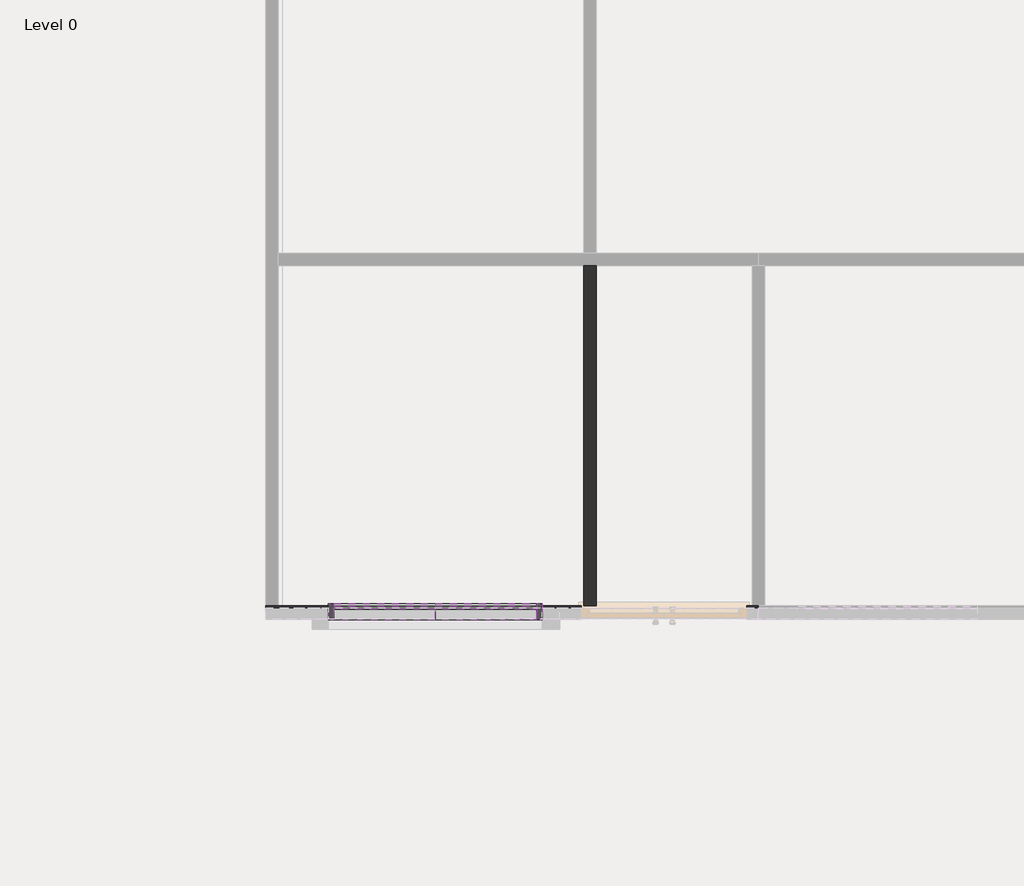
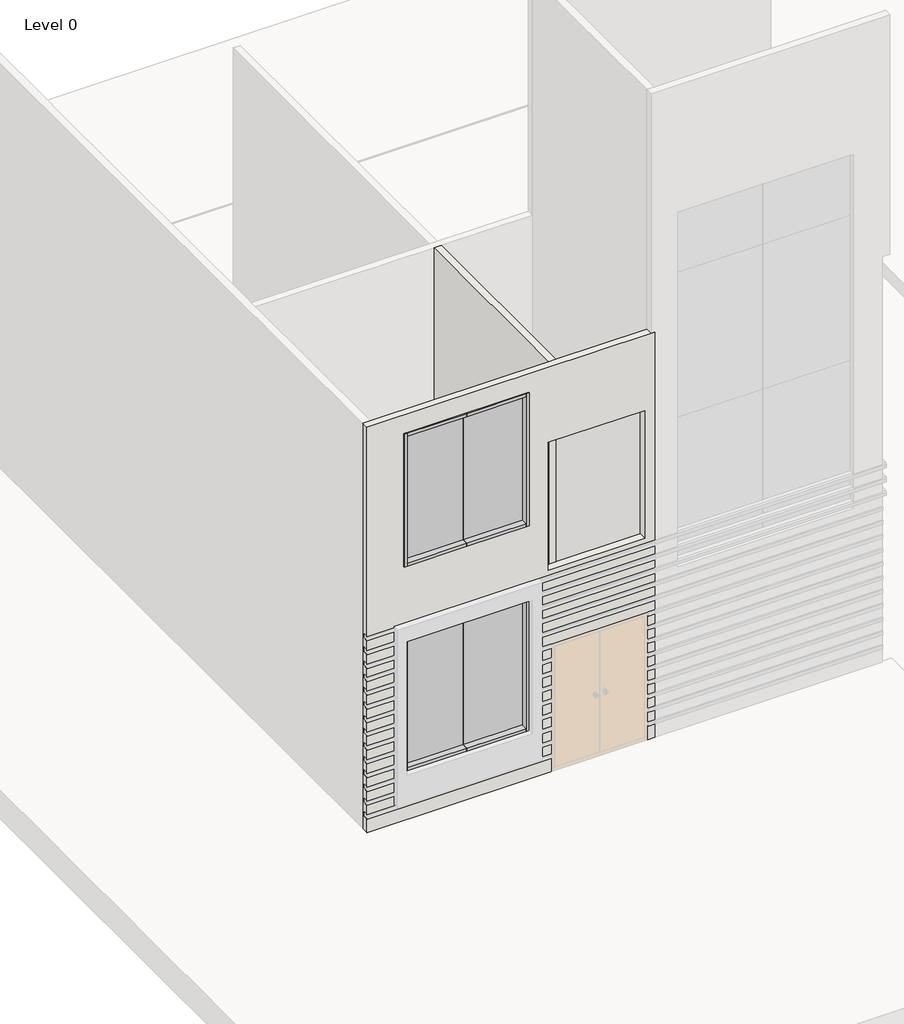
# One storey, part 1 of 5: 30 members, 10 plates, 2 walls.
"""IFC4 building model written with IfcOpenShell, lengths in millimetres."""

from ifc_helpers import new_model, si_unit, origin, origin_with_axes, place, context, project, spatial, polyline, outline, extrude, faceted_brep, transform, mapped, element, save
from components import rectangular_mullion_50x150mm_7233a1e1, rectangular_mullion_50x150mm_68afe020, rectangular_mullion_50x150mm_7f05dd67, system_panel_glazed_63ec7693, system_panel_glazed_65c2c16a

model = new_model("IFC4")

# Units and contexts
model_context = context("Model", 3, world=origin())
ifc_project = project(units=[si_unit("LENGTHUNIT", "METRE", prefix="MILLI")], contexts=[model_context])

# Site, building, storey
site = spatial("IfcSite", under=ifc_project)
building = spatial("IfcBuilding", under=site)
storey = spatial("IfcBuildingStorey", under=building, Name="Level 0", Elevation=0.0)

# Members
placement = place(None, origin())
rectangular_mullion_50x150mm_shape = rectangular_mullion_50x150mm_7233a1e1(model_context)
element("IfcMember", 1, ObjectType="Rectangular Mullion : 50x150mm", at=placement, inside=storey, context=model_context, shape_type="MappedRepresentation", body=[
    mapped(rectangular_mullion_50x150mm_shape, transform((-18841.229089, -2815.8968048, 6400.8), x_axis=(-1.0, 0.0, 0.0), y_axis=(0.0, -1.0, 0.0), z_axis=(0.0, 0.0, 1.0))),
])
element("IfcMember", 2, ObjectType="Rectangular Mullion : 50x150mm", at=placement, inside=storey, context=model_context, shape_type="MappedRepresentation", body=[
    mapped(rectangular_mullion_50x150mm_shape, transform((-18841.229089, -2815.8968048, 6400.8), x_axis=(-1.0, 0.0, 0.0), y_axis=(0.0, -1.0, 0.0), z_axis=(0.0, 0.0, 1.0))),
])
element("IfcMember", 3, ObjectType="Rectangular Mullion : 50x150mm", at=placement, inside=storey, context=model_context, shape_type="MappedRepresentation", body=[
    mapped(rectangular_mullion_50x150mm_shape, transform((-18841.229089, -2815.8968048, 6400.8), x_axis=(-1.0, 0.0, 0.0), y_axis=(0.0, -1.0, 0.0), z_axis=(0.0, 0.0, 1.0))),
])
element("IfcMember", 4, ObjectType="Rectangular Mullion : 50x150mm", at=placement, inside=storey, context=model_context, shape_type="MappedRepresentation", body=[
    mapped(rectangular_mullion_50x150mm_shape, transform((-18841.229089, -2815.8968048, 6400.8), x_axis=(-1.0, 0.0, 0.0), y_axis=(0.0, -1.0, 0.0), z_axis=(0.0, 0.0, 1.0))),
])
element("IfcMember", 5, ObjectType="Rectangular Mullion : 50x150mm", at=placement, inside=storey, context=model_context, shape_type="MappedRepresentation", body=[
    mapped(rectangular_mullion_50x150mm_shape, transform((-16885.429089, -2815.8968048, 4204.0934893), x_axis=(1.0, 0.0, 0.0), y_axis=(0.0, -1.0, 0.0), z_axis=(0.0, 0.0, -1.0))),
])
element("IfcMember", 6, ObjectType="Rectangular Mullion : 50x150mm", at=placement, inside=storey, context=model_context, shape_type="MappedRepresentation", body=[
    mapped(rectangular_mullion_50x150mm_shape, transform((-16885.429089, -2815.8968048, 4204.0934893), x_axis=(1.0, 0.0, 0.0), y_axis=(0.0, -1.0, 0.0), z_axis=(0.0, 0.0, -1.0))),
])
element("IfcMember", 7, ObjectType="Rectangular Mullion : 50x150mm", at=placement, inside=storey, context=model_context, shape_type="MappedRepresentation", body=[
    mapped(rectangular_mullion_50x150mm_shape, transform((-16885.429089, -2815.8968048, 4204.0934893), x_axis=(1.0, 0.0, 0.0), y_axis=(0.0, -1.0, 0.0), z_axis=(0.0, 0.0, -1.0))),
])
element("IfcMember", 8, ObjectType="Rectangular Mullion : 50x150mm", at=placement, inside=storey, context=model_context, shape_type="MappedRepresentation", body=[
    mapped(rectangular_mullion_50x150mm_shape, transform((-16885.429089, -2815.8968048, 4204.0934893), x_axis=(1.0, 0.0, 0.0), y_axis=(0.0, -1.0, 0.0), z_axis=(0.0, 0.0, -1.0))),
])
rectangular_mullion_50x150mm_2_shape = rectangular_mullion_50x150mm_68afe020(model_context)
element("IfcMember", 9, ObjectType="Rectangular Mullion : 50x150mm", at=placement, inside=storey, context=model_context, shape_type="MappedRepresentation", body=[
    mapped(rectangular_mullion_50x150mm_2_shape, transform((-16935.429089, -2815.8968048, 6400.8), x_axis=(0.0, 0.0, 1.0), y_axis=(0.0, -1.0, 0.0), z_axis=(1.0, 0.0, 0.0))),
])
element("IfcMember", 10, ObjectType="Rectangular Mullion : 50x150mm", at=placement, inside=storey, context=model_context, shape_type="MappedRepresentation", body=[
    mapped(rectangular_mullion_50x150mm_2_shape, transform((-16935.429089, -2815.8968048, 6400.8), x_axis=(0.0, 0.0, 1.0), y_axis=(0.0, -1.0, 0.0), z_axis=(1.0, 0.0, 0.0))),
])
element("IfcMember", 11, ObjectType="Rectangular Mullion : 50x150mm", at=placement, inside=storey, context=model_context, shape_type="MappedRepresentation", body=[
    mapped(rectangular_mullion_50x150mm_2_shape, transform((-16935.429089, -2815.8968048, 6400.8), x_axis=(0.0, 0.0, 1.0), y_axis=(0.0, -1.0, 0.0), z_axis=(1.0, 0.0, 0.0))),
])
element("IfcMember", 12, ObjectType="Rectangular Mullion : 50x150mm", at=placement, inside=storey, context=model_context, shape_type="MappedRepresentation", body=[
    mapped(rectangular_mullion_50x150mm_2_shape, transform((-16935.429089, -2815.8968048, 6400.8), x_axis=(0.0, 0.0, 1.0), y_axis=(0.0, -1.0, 0.0), z_axis=(1.0, 0.0, 0.0))),
])
element("IfcMember", 13, ObjectType="Rectangular Mullion : 50x150mm", at=placement, inside=storey, context=model_context, shape_type="MappedRepresentation", body=[
    mapped(rectangular_mullion_50x150mm_2_shape, transform((-16935.429089, -2815.8968048, 3018.6850236), x_axis=(0.0, 0.0, 1.0), y_axis=(0.0, -1.0, 0.0), z_axis=(1.0, 0.0, 0.0))),
])
element("IfcMember", 14, ObjectType="Rectangular Mullion : 50x150mm", at=placement, inside=storey, context=model_context, shape_type="MappedRepresentation", body=[
    mapped(rectangular_mullion_50x150mm_2_shape, transform((-18791.229089, -2815.8968048, 4204.0934893), x_axis=(0.0, 0.0, -1.0), y_axis=(0.0, -1.0, 0.0), z_axis=(-1.0, 0.0, 0.0))),
])
element("IfcMember", 15, ObjectType="Rectangular Mullion : 50x150mm", at=placement, inside=storey, context=model_context, shape_type="MappedRepresentation", body=[
    mapped(rectangular_mullion_50x150mm_2_shape, transform((-18791.229089, -2815.8968048, 4204.0934893), x_axis=(0.0, 0.0, -1.0), y_axis=(0.0, -1.0, 0.0), z_axis=(-1.0, 0.0, 0.0))),
])
element("IfcMember", 16, ObjectType="Rectangular Mullion : 50x150mm", at=placement, inside=storey, context=model_context, shape_type="MappedRepresentation", body=[
    mapped(rectangular_mullion_50x150mm_2_shape, transform((-18791.229089, -2815.8968048, 4204.0934893), x_axis=(0.0, 0.0, -1.0), y_axis=(0.0, -1.0, 0.0), z_axis=(-1.0, 0.0, 0.0))),
])
element("IfcMember", 17, ObjectType="Rectangular Mullion : 50x150mm", at=placement, inside=storey, context=model_context, shape_type="MappedRepresentation", body=[
    mapped(rectangular_mullion_50x150mm_2_shape, transform((-18791.229089, -2815.8968048, 4204.0934893), x_axis=(0.0, 0.0, -1.0), y_axis=(0.0, -1.0, 0.0), z_axis=(-1.0, 0.0, 0.0))),
])
element("IfcMember", 18, ObjectType="Rectangular Mullion : 50x150mm", at=placement, inside=storey, context=model_context, shape_type="MappedRepresentation", body=[
    mapped(rectangular_mullion_50x150mm_2_shape, transform((-18791.229089, -2815.8968048, 815.9706649), x_axis=(0.0, 0.0, -1.0), y_axis=(0.0, -1.0, 0.0), z_axis=(-1.0, 0.0, 0.0))),
])
element("IfcMember", 19, ObjectType="Rectangular Mullion : 50x150mm", at=placement, inside=storey, context=model_context, shape_type="MappedRepresentation", body=[
    mapped(rectangular_mullion_50x150mm_2_shape, transform((-17863.329089, -2815.8968048, 6400.8), x_axis=(0.0, 0.0, 1.0), y_axis=(0.0, -1.0, 0.0), z_axis=(1.0, 0.0, 0.0))),
])
element("IfcMember", 20, ObjectType="Rectangular Mullion : 50x150mm", at=placement, inside=storey, context=model_context, shape_type="MappedRepresentation", body=[
    mapped(rectangular_mullion_50x150mm_2_shape, transform((-17863.329089, -2815.8968048, 6400.8), x_axis=(0.0, 0.0, 1.0), y_axis=(0.0, -1.0, 0.0), z_axis=(1.0, 0.0, 0.0))),
])
element("IfcMember", 21, ObjectType="Rectangular Mullion : 50x150mm", at=placement, inside=storey, context=model_context, shape_type="MappedRepresentation", body=[
    mapped(rectangular_mullion_50x150mm_2_shape, transform((-17863.329089, -2815.8968048, 6400.8), x_axis=(0.0, 0.0, 1.0), y_axis=(0.0, -1.0, 0.0), z_axis=(1.0, 0.0, 0.0))),
])
element("IfcMember", 22, ObjectType="Rectangular Mullion : 50x150mm", at=placement, inside=storey, context=model_context, shape_type="MappedRepresentation", body=[
    mapped(rectangular_mullion_50x150mm_2_shape, transform((-17863.329089, -2815.8968048, 6400.8), x_axis=(0.0, 0.0, 1.0), y_axis=(0.0, -1.0, 0.0), z_axis=(1.0, 0.0, 0.0))),
])
element("IfcMember", 23, ObjectType="Rectangular Mullion : 50x150mm", at=placement, inside=storey, context=model_context, shape_type="MappedRepresentation", body=[
    mapped(rectangular_mullion_50x150mm_2_shape, transform((-17863.329089, -2815.8968048, 3018.6850236), x_axis=(0.0, 0.0, 1.0), y_axis=(0.0, -1.0, 0.0), z_axis=(1.0, 0.0, 0.0))),
])
element("IfcMember", 24, ObjectType="Rectangular Mullion : 50x150mm", at=placement, inside=storey, context=model_context, shape_type="MappedRepresentation", body=[
    mapped(rectangular_mullion_50x150mm_2_shape, transform((-17863.329089, -2815.8968048, 4204.0934893), x_axis=(0.0, 0.0, -1.0), y_axis=(0.0, -1.0, 0.0), z_axis=(-1.0, 0.0, 0.0))),
])
element("IfcMember", 25, ObjectType="Rectangular Mullion : 50x150mm", at=placement, inside=storey, context=model_context, shape_type="MappedRepresentation", body=[
    mapped(rectangular_mullion_50x150mm_2_shape, transform((-17863.329089, -2815.8968048, 4204.0934893), x_axis=(0.0, 0.0, -1.0), y_axis=(0.0, -1.0, 0.0), z_axis=(-1.0, 0.0, 0.0))),
])
element("IfcMember", 26, ObjectType="Rectangular Mullion : 50x150mm", at=placement, inside=storey, context=model_context, shape_type="MappedRepresentation", body=[
    mapped(rectangular_mullion_50x150mm_2_shape, transform((-17863.329089, -2815.8968048, 4204.0934893), x_axis=(0.0, 0.0, -1.0), y_axis=(0.0, -1.0, 0.0), z_axis=(-1.0, 0.0, 0.0))),
])
element("IfcMember", 27, ObjectType="Rectangular Mullion : 50x150mm", at=placement, inside=storey, context=model_context, shape_type="MappedRepresentation", body=[
    mapped(rectangular_mullion_50x150mm_2_shape, transform((-17863.329089, -2815.8968048, 4204.0934893), x_axis=(0.0, 0.0, -1.0), y_axis=(0.0, -1.0, 0.0), z_axis=(-1.0, 0.0, 0.0))),
])
element("IfcMember", 28, ObjectType="Rectangular Mullion : 50x150mm", at=placement, inside=storey, context=model_context, shape_type="MappedRepresentation", body=[
    mapped(rectangular_mullion_50x150mm_2_shape, transform((-17863.329089, -2815.8968048, 815.9706649), x_axis=(0.0, 0.0, -1.0), y_axis=(0.0, -1.0, 0.0), z_axis=(-1.0, 0.0, 0.0))),
])
rectangular_mullion_50x150mm_3_shape = rectangular_mullion_50x150mm_7f05dd67(model_context)
element("IfcMember", 29, ObjectType="Rectangular Mullion : 50x150mm", at=placement, inside=storey, context=model_context, shape_type="MappedRepresentation", body=[
    mapped(rectangular_mullion_50x150mm_3_shape, transform((-18841.229089, -2815.8968048, 3018.6850236), x_axis=(-1.0, 0.0, 0.0), y_axis=(0.0, -1.0, 0.0), z_axis=(0.0, 0.0, 1.0))),
])
element("IfcMember", 30, ObjectType="Rectangular Mullion : 50x150mm", at=placement, inside=storey, context=model_context, shape_type="MappedRepresentation", body=[
    mapped(rectangular_mullion_50x150mm_3_shape, transform((-16885.429089, -2815.8968048, 815.9706649), x_axis=(1.0, 0.0, 0.0), y_axis=(0.0, -1.0, 0.0), z_axis=(0.0, 0.0, -1.0))),
])

# Plates
system_panel_glazed_shape = system_panel_glazed_63ec7693(model_context)
element("IfcPlate", 31, ObjectType="System Panel : Glazed", at=placement, inside=storey, context=model_context, shape_type="MappedRepresentation", body=[
    mapped(system_panel_glazed_shape, transform((-18327.279089, -2815.8968048, 4254.0934893), x_axis=(1.0, 0.0, 0.0), y_axis=(0.0, 1.0, 0.0), z_axis=(0.0, 0.0, 1.0))),
])
element("IfcPlate", 32, ObjectType="System Panel : Glazed", at=placement, inside=storey, context=model_context, shape_type="MappedRepresentation", body=[
    mapped(system_panel_glazed_shape, transform((-17399.379089, -2815.8968048, 4254.0934893), x_axis=(1.0, 0.0, 0.0), y_axis=(0.0, 1.0, 0.0), z_axis=(0.0, 0.0, 1.0))),
])
element("IfcPlate", 33, ObjectType="System Panel : Glazed", at=placement, inside=storey, context=model_context, shape_type="MappedRepresentation", body=[
    mapped(system_panel_glazed_shape, transform((-18327.279089, -2815.8968048, 4254.0934893), x_axis=(1.0, 0.0, 0.0), y_axis=(0.0, 1.0, 0.0), z_axis=(0.0, 0.0, 1.0))),
])
element("IfcPlate", 34, ObjectType="System Panel : Glazed", at=placement, inside=storey, context=model_context, shape_type="MappedRepresentation", body=[
    mapped(system_panel_glazed_shape, transform((-17399.379089, -2815.8968048, 4254.0934893), x_axis=(1.0, 0.0, 0.0), y_axis=(0.0, 1.0, 0.0), z_axis=(0.0, 0.0, 1.0))),
])
element("IfcPlate", 35, ObjectType="System Panel : Glazed", at=placement, inside=storey, context=model_context, shape_type="MappedRepresentation", body=[
    mapped(system_panel_glazed_shape, transform((-18327.279089, -2815.8968048, 4254.0934893), x_axis=(1.0, 0.0, 0.0), y_axis=(0.0, 1.0, 0.0), z_axis=(0.0, 0.0, 1.0))),
])
element("IfcPlate", 36, ObjectType="System Panel : Glazed", at=placement, inside=storey, context=model_context, shape_type="MappedRepresentation", body=[
    mapped(system_panel_glazed_shape, transform((-17399.379089, -2815.8968048, 4254.0934893), x_axis=(1.0, 0.0, 0.0), y_axis=(0.0, 1.0, 0.0), z_axis=(0.0, 0.0, 1.0))),
])
element("IfcPlate", 37, ObjectType="System Panel : Glazed", at=placement, inside=storey, context=model_context, shape_type="MappedRepresentation", body=[
    mapped(system_panel_glazed_shape, transform((-18327.279089, -2815.8968048, 4254.0934893), x_axis=(1.0, 0.0, 0.0), y_axis=(0.0, 1.0, 0.0), z_axis=(0.0, 0.0, 1.0))),
])
element("IfcPlate", 38, ObjectType="System Panel : Glazed", at=placement, inside=storey, context=model_context, shape_type="MappedRepresentation", body=[
    mapped(system_panel_glazed_shape, transform((-17399.379089, -2815.8968048, 4254.0934893), x_axis=(1.0, 0.0, 0.0), y_axis=(0.0, 1.0, 0.0), z_axis=(0.0, 0.0, 1.0))),
])
system_panel_glazed_2_shape = system_panel_glazed_65c2c16a(model_context)
element("IfcPlate", 39, ObjectType="System Panel : Glazed", at=placement, inside=storey, context=model_context, shape_type="MappedRepresentation", body=[
    mapped(system_panel_glazed_2_shape, transform((-18327.279089, -2815.8968048, 865.9706649), x_axis=(1.0, 0.0, 0.0), y_axis=(0.0, 1.0, 0.0), z_axis=(0.0, 0.0, 1.0))),
])
element("IfcPlate", 40, ObjectType="System Panel : Glazed", at=placement, inside=storey, context=model_context, shape_type="MappedRepresentation", body=[
    mapped(system_panel_glazed_2_shape, transform((-17399.379089, -2815.8968048, 865.9706649), x_axis=(1.0, 0.0, 0.0), y_axis=(0.0, 1.0, 0.0), z_axis=(0.0, 0.0, 1.0))),
])

# Walls
element("IfcWall", 41, ObjectType="basic wall", at=placement, inside=storey, context=model_context, shape_type="Brep", body=[
    faceted_brep([(-14910.579089, -2873.0468048, 6705.6), (-14967.729089, -2873.0468048, 6705.6), (-19298.429089, -2873.0468048, 6705.6), (-19412.729089, -2873.0468048, 6705.6), (-19412.729089, -2873.0468048, 3352.8), (-19412.729089, -2873.0468048, 3242.6284072), (-14910.579089, -2873.0468048, 3242.6284072), (-14910.579089, -2873.0468048, 3265.4), (-18841.229089, -2873.0468048, 4204.0934893), (-18841.229089, -2873.0468048, 6400.8), (-16885.429089, -2873.0468048, 6400.8), (-16885.429089, -2873.0468048, 4204.0934893), (-16579.329089, -2873.0468048, 3352.8), (-16579.329089, -2873.0468048, 5462.8), (-15069.329089, -2873.0468048, 5462.8), (-15069.329089, -2873.0468048, 3352.8), (-18841.229089, -2873.0468048, 3018.6850236), (-16885.429089, -2873.0468048, 3018.6850236), (-16885.429089, -2873.0468048, 3014.0284072), (-14910.579089, -2873.0468048, 3014.0284072), (-14910.579089, -2873.0468048, 3036.8), (-14910.579089, -2873.0468048, 3177.6284072), (-19412.729089, -2873.0468048, 3177.6284072), (-19412.729089, -2873.0468048, 3014.0284072), (-18841.229089, -2873.0468048, 3014.0284072), (-16885.429089, -2873.0468048, 815.9706649), (-18841.229089, -2873.0468048, 815.9706649), (-18841.229089, -2873.0468048, 914.4), (-19412.729089, -2873.0468048, 914.4), (-19412.729089, -2873.0468048, 750.8), (-16528.529089, -2873.0468048, 750.8), (-16528.529089, -2873.0468048, 914.4), (-16885.429089, -2873.0468048, 914.4), (-19412.729089, -2873.0468048, 0.0), (-16528.529089, -2873.0468048, 0.0), (-16528.529089, -2873.0468048, 228.6), (-19412.729089, -2873.0468048, 228.6), (-15018.529089, -2873.0468048, 0.0), (-14910.579089, -2873.0468048, 0.0), (-14910.579089, -2873.0468048, 228.6), (-15018.529089, -2873.0468048, 228.6), (-16528.529089, -2873.0468048, 2110.0), (-15018.529089, -2873.0468048, 2110.0), (-15018.529089, -2873.0468048, 2114.6106439), (-14910.579089, -2873.0468048, 2114.6106439), (-14910.579089, -2873.0468048, 2122.4), (-14910.579089, -2873.0468048, 2278.2106439), (-16885.429089, -2873.0468048, 2278.2106439), (-16885.429089, -2873.0468048, 2114.6106439), (-16528.529089, -2873.0468048, 2114.6106439), (-16727.530247, -2873.0468048, 2579.6), (-14910.579089, -2873.0468048, 2579.6), (-14910.579089, -2873.0468048, 2720.4284072), (-16885.429089, -2873.0468048, 2720.4284072), (-16885.429089, -2873.0468048, 2571.8106439), (-16727.530247, -2873.0468048, 2571.8106439), (-16727.530247, -2873.0468048, 2351.0), (-14910.579089, -2873.0468048, 2351.0), (-14910.579089, -2873.0468048, 2506.8106439), (-16885.429089, -2873.0468048, 2506.8106439), (-16885.429089, -2873.0468048, 2343.2106439), (-16727.530247, -2873.0468048, 2343.2106439), (-15018.529089, -2873.0468048, 293.6), (-14910.579089, -2873.0468048, 293.6), (-14910.579089, -2873.0468048, 457.2), (-15018.529089, -2873.0468048, 457.2), (-19412.729089, -2873.0468048, 293.6), (-16528.529089, -2873.0468048, 293.6), (-16528.529089, -2873.0468048, 457.2), (-19412.729089, -2873.0468048, 457.2), (-15018.529089, -2873.0468048, 522.2), (-14910.579089, -2873.0468048, 522.2), (-14910.579089, -2873.0468048, 685.8), (-15018.529089, -2873.0468048, 685.8), (-19412.729089, -2873.0468048, 522.2), (-16528.529089, -2873.0468048, 522.2), (-16528.529089, -2873.0468048, 685.8), (-19412.729089, -2873.0468048, 685.8), (-15018.529089, -2873.0468048, 750.8), (-14910.579089, -2873.0468048, 750.8), (-14910.579089, -2873.0468048, 914.4), (-15018.529089, -2873.0468048, 914.4), (-15018.529089, -2873.0468048, 979.4), (-14910.579089, -2873.0468048, 979.4), (-14910.579089, -2873.0468048, 1143.0), (-15018.529089, -2873.0468048, 1143.0), (-16885.429089, -2873.0468048, 979.4), (-16528.529089, -2873.0468048, 979.4), (-16528.529089, -2873.0468048, 1143.0), (-16885.429089, -2873.0468048, 1143.0), (-19412.729089, -2873.0468048, 979.4), (-18841.229089, -2873.0468048, 979.4), (-18841.229089, -2873.0468048, 1143.0), (-19412.729089, -2873.0468048, 1143.0), (-15018.529089, -2873.0468048, 1208.0), (-14910.579089, -2873.0468048, 1208.0), (-14910.579089, -2873.0468048, 1371.6), (-15018.529089, -2873.0468048, 1371.6), (-16885.429089, -2873.0468048, 1208.0), (-16528.529089, -2873.0468048, 1208.0), (-16528.529089, -2873.0468048, 1371.6), (-16885.429089, -2873.0468048, 1371.6), (-19412.729089, -2873.0468048, 1208.0), (-18841.229089, -2873.0468048, 1208.0), (-18841.229089, -2873.0468048, 1371.6), (-19412.729089, -2873.0468048, 1371.6), (-15018.529089, -2873.0468048, 1436.6), (-14910.579089, -2873.0468048, 1436.6), (-14910.579089, -2873.0468048, 1600.2), (-15018.529089, -2873.0468048, 1600.2), (-16885.429089, -2873.0468048, 1436.6), (-16528.529089, -2873.0468048, 1436.6), (-16528.529089, -2873.0468048, 1600.2), (-16885.429089, -2873.0468048, 1600.2), (-19412.729089, -2873.0468048, 1436.6), (-18841.229089, -2873.0468048, 1436.6), (-18841.229089, -2873.0468048, 1600.2), (-19412.729089, -2873.0468048, 1600.2), (-15018.529089, -2873.0468048, 1665.2), (-14910.579089, -2873.0468048, 1665.2), (-14910.579089, -2873.0468048, 1821.0106439), (-15018.529089, -2873.0468048, 1821.0106439), (-16885.429089, -2873.0468048, 1665.2), (-16528.529089, -2873.0468048, 1665.2), (-16528.529089, -2873.0468048, 1821.0106439), (-16885.429089, -2873.0468048, 1821.0106439), (-19412.729089, -2873.0468048, 1665.2), (-18841.229089, -2873.0468048, 1665.2), (-18841.229089, -2873.0468048, 1821.0106439), (-19412.729089, -2873.0468048, 1821.0106439), (-15018.529089, -2873.0468048, 1886.0106439), (-14910.579089, -2873.0468048, 1886.0106439), (-14910.579089, -2873.0468048, 1893.8), (-14910.579089, -2873.0468048, 2049.6106439), (-15018.529089, -2873.0468048, 2049.6106439), (-16885.429089, -2873.0468048, 1886.0106439), (-16528.529089, -2873.0468048, 1886.0106439), (-16528.529089, -2873.0468048, 2049.6106439), (-16885.429089, -2873.0468048, 2049.6106439), (-19412.729089, -2873.0468048, 1886.0106439), (-18841.229089, -2873.0468048, 1886.0106439), (-18841.229089, -2873.0468048, 2049.6106439), (-19412.729089, -2873.0468048, 2049.6106439), (-19412.729089, -2873.0468048, 2114.6106439), (-18841.229089, -2873.0468048, 2114.6106439), (-18841.229089, -2873.0468048, 2278.2106439), (-19412.729089, -2873.0468048, 2278.2106439), (-19412.729089, -2873.0468048, 2343.2106439), (-18841.229089, -2873.0468048, 2343.2106439), (-18841.229089, -2873.0468048, 2506.8106439), (-19412.729089, -2873.0468048, 2506.8106439), (-19412.729089, -2873.0468048, 2571.8106439), (-18841.229089, -2873.0468048, 2571.8106439), (-18841.229089, -2873.0468048, 2720.4284072), (-19412.729089, -2873.0468048, 2720.4284072), (-19412.729089, -2873.0468048, 2785.4284072), (-18841.229089, -2873.0468048, 2785.4284072), (-18841.229089, -2873.0468048, 2949.0284072), (-19412.729089, -2873.0468048, 2949.0284072), (-14910.579089, -2873.0468048, 2785.4284072), (-14910.579089, -2873.0468048, 2808.2), (-14910.579089, -2873.0468048, 2949.0284072), (-16885.429089, -2873.0468048, 2949.0284072), (-16885.429089, -2873.0468048, 2785.4284072), (-14910.579089, -2758.7468048, 6705.6), (-14910.579089, -2758.7468048, 0.0), (-14967.729089, -2758.7468048, 0.0), (-15018.529089, -2758.7468048, 0.0), (-15018.529089, -2758.7468048, 2110.0), (-16528.529089, -2758.7468048, 2110.0), (-16528.529089, -2758.7468048, 0.0), (-19298.429089, -2758.7468048, 0.0), (-19412.729089, -2758.7468048, 0.0), (-19412.729089, -2758.7468048, 6705.6), (-19298.429089, -2758.7468048, 6705.6), (-16504.429089, -2758.7468048, 6705.6), (-16390.129089, -2758.7468048, 6705.6), (-14967.729089, -2758.7468048, 6705.6), (-18841.229089, -2758.7468048, 6400.8), (-18841.229089, -2758.7468048, 4204.0934893), (-16885.429089, -2758.7468048, 4204.0934893), (-16885.429089, -2758.7468048, 6400.8), (-18841.229089, -2758.7468048, 3018.6850236), (-18841.229089, -2758.7468048, 815.9706649), (-16885.429089, -2758.7468048, 815.9706649), (-16885.429089, -2758.7468048, 3018.6850236), (-16579.329089, -2758.7468048, 5462.8), (-16579.329089, -2758.7468048, 3352.8), (-15069.329089, -2758.7468048, 3352.8), (-15069.329089, -2758.7468048, 5462.8), (-14910.579089, -2863.0468048, 3252.6284072), (-14910.579089, -2780.5468048, 3252.6284072), (-14910.579089, -2780.5468048, 3177.6284072), (-14910.579089, -2863.0468048, 3024.0284072), (-14910.579089, -2780.5468048, 3024.0284072), (-14910.579089, -2780.5468048, 2949.0284072), (-14910.579089, -2863.0468048, 2795.4284072), (-14910.579089, -2780.5468048, 2795.4284072), (-14910.579089, -2780.5468048, 2720.4284072), (-14910.579089, -2863.0468048, 2589.6), (-14910.579089, -2780.5468048, 2589.6), (-14910.579089, -2780.5468048, 2514.6), (-14910.579089, -2780.5468048, 2506.8106439), (-14910.579089, -2863.0468048, 2361.0), (-14910.579089, -2780.5468048, 2361.0), (-14910.579089, -2780.5468048, 2286.0), (-14910.579089, -2780.5468048, 2278.2106439), (-14910.579089, -2863.0468048, 2124.6106439), (-14910.579089, -2780.5468048, 2124.6106439), (-14910.579089, -2780.5468048, 2057.4), (-14910.579089, -2780.5468048, 2049.6106439), (-14910.579089, -2863.0468048, 1896.0106439), (-14910.579089, -2780.5468048, 1896.0106439), (-14910.579089, -2780.5468048, 1828.8), (-14910.579089, -2780.5468048, 1821.0106439), (-14910.579089, -2863.0468048, 1675.2), (-14910.579089, -2780.5468048, 1675.2), (-14910.579089, -2780.5468048, 1600.2), (-14910.579089, -2863.0468048, 1446.6), (-14910.579089, -2780.5468048, 1446.6), (-14910.579089, -2780.5468048, 1371.6), (-14910.579089, -2863.0468048, 1218.0), (-14910.579089, -2780.5468048, 1218.0), (-14910.579089, -2780.5468048, 1143.0), (-14910.579089, -2863.0468048, 989.4), (-14910.579089, -2780.5468048, 989.4), (-14910.579089, -2780.5468048, 914.4), (-14910.579089, -2863.0468048, 760.8), (-14910.579089, -2780.5468048, 760.8), (-14910.579089, -2780.5468048, 685.8), (-14910.579089, -2863.0468048, 532.2), (-14910.579089, -2780.5468048, 532.2), (-14910.579089, -2780.5468048, 457.2), (-14910.579089, -2863.0468048, 303.6), (-14910.579089, -2780.5468048, 303.6), (-14910.579089, -2780.5468048, 228.6), (-19412.729089, -2780.5468048, 228.6), (-19412.729089, -2780.5468048, 303.6), (-19412.729089, -2863.0468048, 303.6), (-19412.729089, -2780.5468048, 457.2), (-19412.729089, -2780.5468048, 532.2), (-19412.729089, -2863.0468048, 532.2), (-19412.729089, -2780.5468048, 685.8), (-19412.729089, -2780.5468048, 760.8), (-19412.729089, -2863.0468048, 760.8), (-19412.729089, -2780.5468048, 914.4), (-19412.729089, -2780.5468048, 989.4), (-19412.729089, -2863.0468048, 989.4), (-19412.729089, -2780.5468048, 1143.0), (-19412.729089, -2780.5468048, 1218.0), (-19412.729089, -2863.0468048, 1218.0), (-19412.729089, -2780.5468048, 1371.6), (-19412.729089, -2780.5468048, 1446.6), (-19412.729089, -2863.0468048, 1446.6), (-19412.729089, -2780.5468048, 1600.2), (-19412.729089, -2780.5468048, 1675.2), (-19412.729089, -2863.0468048, 1675.2), (-19412.729089, -2780.5468048, 1821.0106439), (-19412.729089, -2780.5468048, 1896.0106439), (-19412.729089, -2863.0468048, 1896.0106439), (-19412.729089, -2780.5468048, 2049.6106439), (-19412.729089, -2780.5468048, 2124.6106439), (-19412.729089, -2863.0468048, 2124.6106439), (-19412.729089, -2780.5468048, 2278.2106439), (-19412.729089, -2780.5468048, 2353.2106439), (-19412.729089, -2863.0468048, 2353.2106439), (-19412.729089, -2780.5468048, 2506.8106439), (-19412.729089, -2780.5468048, 2581.8106439), (-19412.729089, -2863.0468048, 2581.8106439), (-19412.729089, -2780.5468048, 2720.4284072), (-19412.729089, -2780.5468048, 2795.4284072), (-19412.729089, -2863.0468048, 2795.4284072), (-19412.729089, -2780.5468048, 2949.0284072), (-19412.729089, -2780.5468048, 3024.0284072), (-19412.729089, -2863.0468048, 3024.0284072), (-19412.729089, -2780.5468048, 3177.6284072), (-19412.729089, -2780.5468048, 3252.6284072), (-19412.729089, -2863.0468048, 3252.6284072), (-18841.229089, -2780.5468048, 3018.6850236), (-18841.229089, -2780.5468048, 2949.0284072), (-18841.229089, -2863.0468048, 2795.4284072), (-18841.229089, -2780.5468048, 2795.4284072), (-18841.229089, -2780.5468048, 2720.4284072), (-18841.229089, -2863.0468048, 2581.8106439), (-18841.229089, -2780.5468048, 2581.8106439), (-18841.229089, -2780.5468048, 2506.8106439), (-18841.229089, -2863.0468048, 2353.2106439), (-18841.229089, -2780.5468048, 2353.2106439), (-18841.229089, -2780.5468048, 2278.2106439), (-18841.229089, -2863.0468048, 2124.6106439), (-18841.229089, -2780.5468048, 2124.6106439), (-18841.229089, -2780.5468048, 2049.6106439), (-18841.229089, -2863.0468048, 1896.0106439), (-18841.229089, -2780.5468048, 1896.0106439), (-18841.229089, -2780.5468048, 1821.0106439), (-18841.229089, -2863.0468048, 1675.2), (-18841.229089, -2780.5468048, 1675.2), (-18841.229089, -2780.5468048, 1600.2), (-18841.229089, -2863.0468048, 1446.6), (-18841.229089, -2780.5468048, 1446.6), (-18841.229089, -2780.5468048, 1371.6), (-18841.229089, -2863.0468048, 1218.0), (-18841.229089, -2780.5468048, 1218.0), (-18841.229089, -2780.5468048, 1143.0), (-18841.229089, -2863.0468048, 989.4), (-18841.229089, -2780.5468048, 989.4), (-18841.229089, -2780.5468048, 914.4), (-18841.229089, -2868.3901884, 3018.6850236), (-16885.429089, -2780.5468048, 3018.6850236), (-16885.429089, -2868.3901884, 3018.6850236), (-16885.429089, -2780.5468048, 914.4), (-16885.429089, -2780.5468048, 989.4), (-16885.429089, -2863.0468048, 989.4), (-16885.429089, -2780.5468048, 1143.0), (-16885.429089, -2780.5468048, 1218.0), (-16885.429089, -2863.0468048, 1218.0), (-16885.429089, -2780.5468048, 1371.6), (-16885.429089, -2780.5468048, 1446.6), (-16885.429089, -2863.0468048, 1446.6), (-16885.429089, -2780.5468048, 1600.2), (-16885.429089, -2780.5468048, 1675.2), (-16885.429089, -2863.0468048, 1675.2), (-16885.429089, -2780.5468048, 1821.0106439), (-16885.429089, -2780.5468048, 1896.0106439), (-16885.429089, -2863.0468048, 1896.0106439), (-16885.429089, -2780.5468048, 2049.6106439), (-16885.429089, -2780.5468048, 2124.6106439), (-16885.429089, -2863.0468048, 2124.6106439), (-16885.429089, -2780.5468048, 2278.2106439), (-16885.429089, -2780.5468048, 2353.2106439), (-16885.429089, -2863.0468048, 2353.2106439), (-16885.429089, -2780.5468048, 2506.8106439), (-16885.429089, -2780.5468048, 2581.8106439), (-16885.429089, -2863.0468048, 2581.8106439), (-16885.429089, -2780.5468048, 2720.4284072), (-16885.429089, -2780.5468048, 2795.4284072), (-16885.429089, -2863.0468048, 2795.4284072), (-16885.429089, -2780.5468048, 2949.0284072), (-16528.529089, -2780.5468048, 2110.0), (-16528.529089, -2780.5468048, 2049.6106439), (-16528.529089, -2863.0468048, 1896.0106439), (-16528.529089, -2780.5468048, 1896.0106439), (-16528.529089, -2780.5468048, 1821.0106439), (-16528.529089, -2863.0468048, 1675.2), (-16528.529089, -2780.5468048, 1675.2), (-16528.529089, -2780.5468048, 1600.2), (-16528.529089, -2863.0468048, 1446.6), (-16528.529089, -2780.5468048, 1446.6), (-16528.529089, -2780.5468048, 1371.6), (-16528.529089, -2863.0468048, 1218.0), (-16528.529089, -2780.5468048, 1218.0), (-16528.529089, -2780.5468048, 1143.0), (-16528.529089, -2863.0468048, 989.4), (-16528.529089, -2780.5468048, 989.4), (-16528.529089, -2780.5468048, 914.4), (-16528.529089, -2863.0468048, 760.8), (-16528.529089, -2780.5468048, 760.8), (-16528.529089, -2780.5468048, 685.8), (-16528.529089, -2863.0468048, 532.2), (-16528.529089, -2780.5468048, 532.2), (-16528.529089, -2780.5468048, 457.2), (-16528.529089, -2863.0468048, 303.6), (-16528.529089, -2780.5468048, 303.6), (-16528.529089, -2780.5468048, 228.6), (-15018.529089, -2780.5468048, 228.6), (-15018.529089, -2780.5468048, 303.6), (-15018.529089, -2863.0468048, 303.6), (-15018.529089, -2780.5468048, 457.2), (-15018.529089, -2780.5468048, 532.2), (-15018.529089, -2863.0468048, 532.2), (-15018.529089, -2780.5468048, 685.8), (-15018.529089, -2780.5468048, 760.8), (-15018.529089, -2863.0468048, 760.8), (-15018.529089, -2780.5468048, 914.4), (-15018.529089, -2780.5468048, 989.4), (-15018.529089, -2863.0468048, 989.4), (-15018.529089, -2780.5468048, 1143.0), (-15018.529089, -2780.5468048, 1218.0), (-15018.529089, -2863.0468048, 1218.0), (-15018.529089, -2780.5468048, 1371.6), (-15018.529089, -2780.5468048, 1446.6), (-15018.529089, -2863.0468048, 1446.6), (-15018.529089, -2780.5468048, 1600.2), (-15018.529089, -2780.5468048, 1675.2), (-15018.529089, -2863.0468048, 1675.2), (-15018.529089, -2780.5468048, 1821.0106439), (-15018.529089, -2780.5468048, 1896.0106439), (-15018.529089, -2863.0468048, 1896.0106439), (-15018.529089, -2780.5468048, 2049.6106439), (-15018.529089, -2780.5468048, 2110.0), (-16727.530247, -2780.5468048, 2361.0), (-16727.530247, -2863.0468048, 2361.0), (-16727.530247, -2863.0468048, 2353.2106439), (-16727.530247, -2780.5468048, 2353.2106439), (-16727.530247, -2780.5468048, 2589.6), (-16727.530247, -2863.0468048, 2589.6), (-16727.530247, -2863.0468048, 2581.8106439), (-16727.530247, -2780.5468048, 2581.8106439), (-15018.529089, -2780.5468048, 2124.6106439), (-15018.529089, -2863.0468048, 2124.6106439), (-16528.529089, -2863.0468048, 2124.6106439), (-16528.529089, -2780.5468048, 2124.6106439), (-16885.429089, -2780.5468048, 3024.0284072), (-16885.429089, -2863.0468048, 3024.0284072), (-18841.229089, -2863.0468048, 3024.0284072), (-18841.229089, -2780.5468048, 3024.0284072)], [[[0, 1, 2, 3, 4, 5, 6, 7], [8, 9, 10, 11], [12, 13, 14, 15]], [[16, 17, 18, 19, 20, 21, 22, 23, 24]], [[25, 26, 27, 28, 29, 30, 31, 32]], [[33, 34, 35, 36]], [[37, 38, 39, 40]], [[41, 42, 43, 44, 45, 46, 47, 48, 49]], [[50, 51, 52, 53, 54, 55]], [[56, 57, 58, 59, 60, 61]], [[62, 63, 64, 65]], [[66, 67, 68, 69]], [[70, 71, 72, 73]], [[74, 75, 76, 77]], [[78, 79, 80, 81]], [[82, 83, 84, 85]], [[86, 87, 88, 89]], [[90, 91, 92, 93]], [[94, 95, 96, 97]], [[98, 99, 100, 101]], [[102, 103, 104, 105]], [[106, 107, 108, 109]], [[110, 111, 112, 113]], [[114, 115, 116, 117]], [[118, 119, 120, 121]], [[122, 123, 124, 125]], [[126, 127, 128, 129]], [[130, 131, 132, 133, 134]], [[135, 136, 137, 138]], [[139, 140, 141, 142]], [[143, 144, 145, 146]], [[147, 148, 149, 150]], [[151, 152, 153, 154]], [[155, 156, 157, 158]], [[159, 160, 161, 162, 163]], [[164, 165, 166, 167, 168, 169, 170, 171, 172, 173, 174, 175, 176, 177], [178, 179, 180, 181], [182, 183, 184, 185], [186, 187, 188, 189]], [[33, 172, 171, 170, 34]], [[165, 38, 37, 167, 166]], [[165, 164, 0, 7, 6, 190, 191, 192, 21, 20, 19, 193, 194, 195, 161, 160, 159, 196, 197, 198, 52, 51, 199, 200, 201, 202, 58, 57, 203, 204, 205, 206, 46, 45, 44, 207, 208, 209, 210, 133, 132, 131, 211, 212, 213, 214, 120, 119, 215, 216, 217, 108, 107, 218, 219, 220, 96, 95, 221, 222, 223, 84, 83, 224, 225, 226, 80, 79, 227, 228, 229, 72, 71, 230, 231, 232, 64, 63, 233, 234, 235, 39, 38]], [[3, 2, 1, 0, 164, 177, 176, 175, 174, 173]], [[3, 173, 172, 33, 36, 236, 237, 238, 66, 69, 239, 240, 241, 74, 77, 242, 243, 244, 29, 28, 245, 246, 247, 90, 93, 248, 249, 250, 102, 105, 251, 252, 253, 114, 117, 254, 255, 256, 126, 129, 257, 258, 259, 139, 142, 260, 261, 262, 143, 146, 263, 264, 265, 147, 150, 266, 267, 268, 151, 154, 269, 270, 271, 155, 158, 272, 273, 274, 23, 22, 275, 276, 277, 5, 4]], [[8, 179, 178, 9]], [[9, 178, 181, 10]], [[10, 181, 180, 11]], [[179, 8, 11, 180]], [[26, 183, 182, 278, 279, 157, 156, 280, 281, 282, 153, 152, 283, 284, 285, 149, 148, 286, 287, 288, 145, 144, 289, 290, 291, 141, 140, 292, 293, 294, 128, 127, 295, 296, 297, 116, 115, 298, 299, 300, 104, 103, 301, 302, 303, 92, 91, 304, 305, 306, 27]], [[16, 24, 307]], [[17, 16, 307, 278, 182, 185, 308, 309]], [[184, 25, 32, 310, 311, 312, 86, 89, 313, 314, 315, 98, 101, 316, 317, 318, 110, 113, 319, 320, 321, 122, 125, 322, 323, 324, 135, 138, 325, 326, 327, 48, 47, 328, 329, 330, 60, 59, 331, 332, 333, 54, 53, 334, 335, 336, 163, 162, 337, 308, 185]], [[18, 17, 309]], [[183, 26, 25, 184]], [[170, 169, 338, 339, 137, 136, 340, 341, 342, 124, 123, 343, 344, 345, 112, 111, 346, 347, 348, 100, 99, 349, 350, 351, 88, 87, 352, 353, 354, 31, 30, 355, 356, 357, 76, 75, 358, 359, 360, 68, 67, 361, 362, 363, 35, 34]], [[168, 167, 37, 40, 364, 365, 366, 62, 65, 367, 368, 369, 70, 73, 370, 371, 372, 78, 81, 373, 374, 375, 82, 85, 376, 377, 378, 94, 97, 379, 380, 381, 106, 109, 382, 383, 384, 118, 121, 385, 386, 387, 130, 134, 388, 389]], [[42, 41, 338, 169, 168, 389]], [[187, 186, 13, 12]], [[188, 187, 12, 15]], [[189, 188, 15, 14]], [[186, 189, 14, 13]], [[390, 391, 56, 61, 392, 393]], [[56, 391, 203, 57]], [[391, 390, 204, 203]], [[204, 390, 393, 329, 328, 206, 205]], [[394, 395, 50, 55, 396, 397]], [[50, 395, 199, 51]], [[395, 394, 200, 199]], [[200, 394, 397, 332, 331, 202, 201]], [[235, 364, 40, 39]], [[366, 233, 63, 62]], [[233, 366, 365, 234]], [[364, 235, 234, 365]], [[363, 236, 36, 35]], [[238, 361, 67, 66]], [[361, 238, 237, 362]], [[236, 363, 362, 237]], [[232, 367, 65, 64]], [[369, 230, 71, 70]], [[230, 369, 368, 231]], [[367, 232, 231, 368]], [[360, 239, 69, 68]], [[241, 358, 75, 74]], [[358, 241, 240, 359]], [[239, 360, 359, 240]], [[229, 370, 73, 72]], [[372, 227, 79, 78]], [[227, 372, 371, 228]], [[370, 229, 228, 371]], [[357, 242, 77, 76]], [[244, 355, 30, 29]], [[355, 244, 243, 356]], [[242, 357, 356, 243]], [[226, 373, 81, 80]], [[375, 224, 83, 82]], [[224, 375, 374, 225]], [[373, 226, 225, 374]], [[354, 310, 32, 31]], [[312, 352, 87, 86]], [[352, 312, 311, 353]], [[310, 354, 353, 311]], [[306, 245, 28, 27]], [[247, 304, 91, 90]], [[304, 247, 246, 305]], [[245, 306, 305, 246]], [[223, 376, 85, 84]], [[378, 221, 95, 94]], [[221, 378, 377, 222]], [[376, 223, 222, 377]], [[351, 313, 89, 88]], [[315, 349, 99, 98]], [[349, 315, 314, 350]], [[313, 351, 350, 314]], [[303, 248, 93, 92]], [[250, 301, 103, 102]], [[301, 250, 249, 302]], [[248, 303, 302, 249]], [[220, 379, 97, 96]], [[381, 218, 107, 106]], [[218, 381, 380, 219]], [[379, 220, 219, 380]], [[348, 316, 101, 100]], [[318, 346, 111, 110]], [[346, 318, 317, 347]], [[316, 348, 347, 317]], [[300, 251, 105, 104]], [[253, 298, 115, 114]], [[298, 253, 252, 299]], [[251, 300, 299, 252]], [[217, 382, 109, 108]], [[384, 215, 119, 118]], [[215, 384, 383, 216]], [[382, 217, 216, 383]], [[345, 319, 113, 112]], [[321, 343, 123, 122]], [[343, 321, 320, 344]], [[319, 345, 344, 320]], [[297, 254, 117, 116]], [[256, 295, 127, 126]], [[295, 256, 255, 296]], [[254, 297, 296, 255]], [[214, 385, 121, 120]], [[387, 211, 131, 130]], [[211, 387, 386, 212]], [[385, 214, 213, 212, 386]], [[342, 322, 125, 124]], [[324, 340, 136, 135]], [[340, 324, 323, 341]], [[322, 342, 341, 323]], [[294, 257, 129, 128]], [[259, 292, 140, 139]], [[292, 259, 258, 293]], [[257, 294, 293, 258]], [[398, 399, 43, 42, 389]], [[210, 388, 134, 133]], [[399, 207, 44, 43]], [[399, 398, 208, 207]], [[388, 210, 209, 208, 398, 389]], [[400, 401, 338, 41, 49]], [[339, 325, 138, 137]], [[327, 400, 49, 48]], [[401, 400, 327, 326]], [[325, 339, 338, 401, 326]], [[291, 260, 142, 141]], [[262, 289, 144, 143]], [[289, 262, 261, 290]], [[260, 291, 290, 261]], [[206, 328, 47, 46]], [[330, 392, 61, 60]], [[329, 393, 392, 330]], [[288, 263, 146, 145]], [[265, 286, 148, 147]], [[286, 265, 264, 287]], [[263, 288, 287, 264]], [[202, 331, 59, 58]], [[333, 396, 55, 54]], [[332, 397, 396, 333]], [[285, 266, 150, 149]], [[268, 283, 152, 151]], [[283, 268, 267, 284]], [[266, 285, 284, 267]], [[198, 334, 53, 52]], [[336, 196, 159, 163]], [[196, 336, 335, 197]], [[334, 198, 197, 335]], [[282, 269, 154, 153]], [[271, 280, 156, 155]], [[280, 271, 270, 281]], [[269, 282, 281, 270]], [[402, 403, 309, 308]], [[195, 337, 162, 161]], [[403, 193, 19, 18, 309]], [[403, 402, 194, 193]], [[337, 195, 194, 402, 308]], [[404, 405, 278, 307]], [[279, 272, 158, 157]], [[274, 404, 307, 24, 23]], [[405, 404, 274, 273]], [[272, 279, 278, 405, 273]], [[192, 275, 22, 21]], [[277, 190, 6, 5]], [[190, 277, 276, 191]], [[275, 192, 191, 276]]]),
])
element("IfcWall", 42, ObjectType="basic wall", at=placement, inside=storey, context=model_context, shape_type="SweptSolid", body=[
    extrude(outline(polyline([(-16504.429089, -2758.7468048), (-16504.429089, 346.4031952), (-16390.129089, 346.4031952), (-16390.129089, -2758.7468048), (-16504.429089, -2758.7468048)])), origin_with_axes(), (0.0, 0.0, 1.0), 6705.6),
])

save(model, "model.ifc")

# Revit data of these elements
# Type "Rectangular Mullion : 50x150mm"
#   Keynote = "H11"
#   built-in parameter 1007304 = 0.492126 (stored number, unit not read)
#   built-in parameter 1007301 = 0.082021 (stored number, unit not read)
#   built-in parameter 1007300 = 0.082021 (stored number, unit not read)
# Type "System Panel : Glazed"
#   Keynote = "H11"
#   Construction Type Id = "GSP4R"
#   Analytic Construction = "1/8 in Pilkington single glazing"
#   Visual Light Transmittance = 0.9
#   Solar Heat Gain Coefficient = 0.86
#   Heat Transfer Coefficient (U) = 6.7069 W/(m²·K)
#   Define Thermal Properties by = 1
# Type "basic wall"
#   Keynote = "F10"
#   Layers, outside or top first: 0' - 4 1/2" "Air" (function 1)
# Elements 1, 2, 3, 4, 5, 6, 7, 8, 9, 10, 11, 12, 13, 14, 15, 16, 17, 18, 19, 20, 21, 22, 23, 24, 25, 26, 27, 28, 29, 30 (IfcMember, "Rectangular Mullion : 50x150mm")
#   Phase Created = New Construction
#   Materials on its faces: "Aluminium"
# Elements 31, 32, 33, 34, 35, 36, 37, 38, 39, 40 (IfcPlate, "System Panel : Glazed")
#   Phase Created = New Construction
#   Materials on its faces: "Glass"
# Elements 41, 42 (IfcWall, "basic wall")
#   Top Offset = 0' - 0"
#   Base Offset = 0' - 0"
#   wall height = 22' - 0"
#   Phase Created = New Construction
#   Base Constraint = Level 0
#   Top Constraint = Level 2
#   Materials on its faces: "Air"
# Materials
#   "Air": class "Gas", colour RGB 255 255 255, transparency 0, Description = "Air", Cost = 0
#   "Aluminium": class "Metal", colour RGB 247 247 247, transparency 0, Description = "Aluminium 6061", Cost = 0
#   "Glass": class "Glass", colour RGB 0 128 192, transparency 0.9, Description = "Soda Lime Glass", Cost = 0
